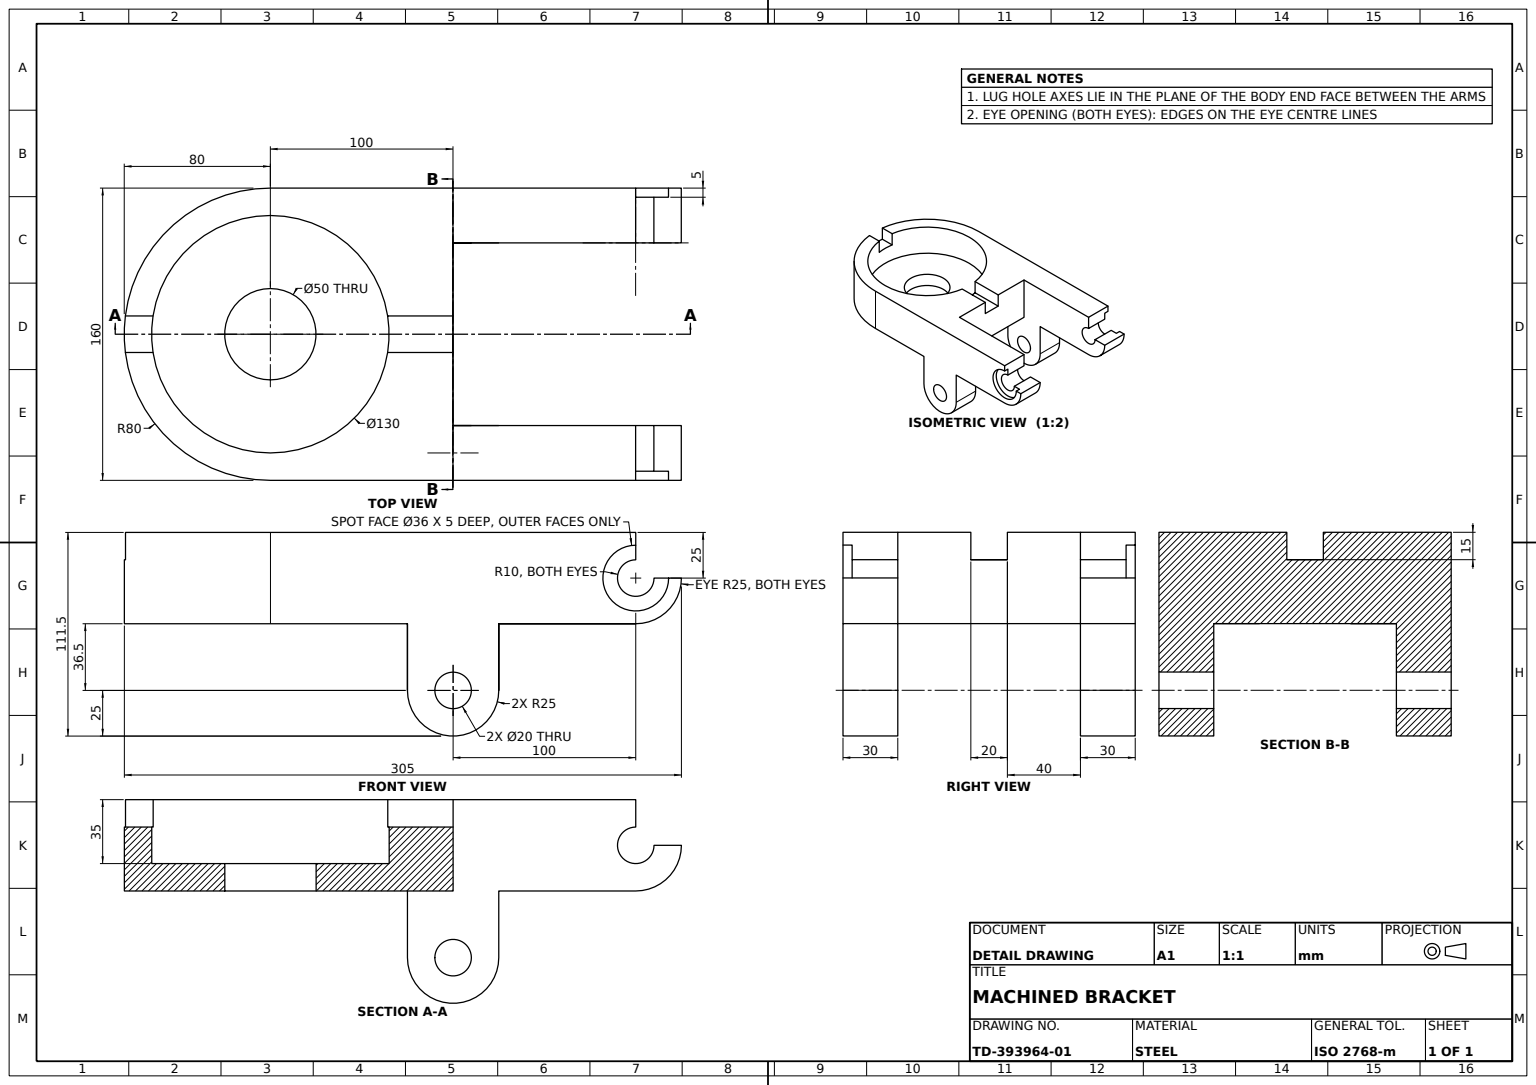
from build123d import *
from build123d.topology import SkipClean

# Parameters (mm, degrees)
BASE_PLATE_DEPTH                = 15
CIRCULAR_START                  = 35
CIRCULAR_HOUSING_DEPTH          = 35
HOUSING_EXTENSION_SKETCH_R      = 65
HOUSING_EXTENSION_SKETCH_R_2    = 25
HOUSING_EXTENSION_DEPTH         = 15
CLEVIS_LUG_BLOCK_SKETCH_R       = 25
CLEVIS_LUG_BLOCK_SKETCH_R_2     = 10
CLEVIS_LUG_BLOCK_DEPTH          = 30
CLEVIS_START                    = -30
CLEVIS_LUG_EXTENSION_SKETCH_R   = 25
CLEVIS_LUG_EXTENSION_SKETCH_R_2 = 10
CLEVIS_LUG_EXTENSION_DEPTH      = 30
PIVOT_LUG_SKETCH_R              = 25
PIVOT_LUGS_DEPTH                = 30
PIVOT_PIN_HOLE_SKETCH_R         = 10
PIVOT_PIN_HOLE_20_DEPTH         = 200
CLEVIS_SLOT_25_DEPTH            = 200
SPOT_FACE_A_SKETCH_R            = 18
SPOT_FACE_A_36X5_DEPTH          = 5
LUG_START                       = -30
LUG_FILL_BOSS_DEPTH             = 30
SPOT_START                      = -5
SPOT_FACE_B_SKETCH_R            = 18
SPOT_FACE_B_36X5_DEPTH          = 5


with BuildPart() as part:
    # Base Plate Sketch → Base Plate (new body)
    with BuildSketch(Plane(origin=(0, 0, 0), x_dir=(1, 0, 0), z_dir=(0, 1, 0))):
        with BuildLine():
            ThreePointArc((64.226162893, -10), (0, -65), (-64.226162893, -10))
            Line((-64.226162893, -10), (-79.372539332, -10))
            ThreePointArc((-79.372539332, -10), (-52.915026221, -60), (0, -80))
            ThreePointArc((0, -80), (52.915026221, -60), (79.372539332, -10))
            Line((79.372539332, -10), (64.226162893, -10))
        make_face()
        with BuildLine():
            ThreePointArc((0, 80), (-52.915026221, 60), (-79.372539332, 10))
            Line((-79.372539332, 10), (-64.226162893, 10))
            ThreePointArc((-64.226162893, 10), (0, 65), (64.226162893, 10))
            Line((64.226162893, 10), (79.372539332, 10))
            ThreePointArc((79.372539332, 10), (52.915026221, 60), (0, 80))
        make_face()
        with BuildLine():
            Line((200, 80), (0, 80))
            ThreePointArc((0, 80), (52.915026221, 60), (79.372539332, 10))
            Line((79.372539332, 10), (100, 10))
            Line((100, 10), (100, 50))
            Line((100, 50), (200, 50))
            Line((200, 50), (200, 80))
        make_face()
        with BuildLine():
            ThreePointArc((79.372539332, -10), (52.915026221, -60), (0, -80))
            Line((0, -80), (200, -80))
            Line((200, -80), (200, -50))
            Line((200, -50), (100, -50))
            Line((100, -50), (100, -10))
            Line((100, -10), (79.372539332, -10))
        make_face()
    extrude(amount=BASE_PLATE_DEPTH)

    # Circular Housing Sketch → Circular Housing (add)
    with BuildSketch(Plane.XZ.offset(CIRCULAR_START)):
        with BuildLine():
            ThreePointArc((79.372539332, 10), (52.915026221, 60), (0, 80))
            ThreePointArc((0, 80), (-52.915026221, 60), (-79.372539332, 10))
            Line((-79.372539332, 10), (-64.226162893, 10))
            ThreePointArc((-64.226162893, 10), (0, 65), (64.226162893, 10))
            Line((64.226162893, 10), (79.372539332, 10))
        make_face()
        with BuildLine():
            Line((-64.226162893, 10), (-79.372539332, 10))
            ThreePointArc((-79.372539332, 10), (-60, -52.915026221), (0, -80))
            ThreePointArc((0, -80), (56.568542495, -56.568542495), (80, 0))
            ThreePointArc((80, 0), (79.842980739, 5.009833003), (79.372539332, 10))
            Line((79.372539332, 10), (64.226162893, 10))
            ThreePointArc((64.226162893, 10), (64.806251967, 5.014948252), (65, 0))
            ThreePointArc((65, 0), (-5.014948252, -64.806251967), (-64.226162893, 10))
        make_face()
        with BuildLine():
            Line((200, 80), (0, 80))
            ThreePointArc((0, 80), (52.915026221, 60), (79.372539332, 10))
            Line((79.372539332, 10), (100, 10))
            Line((100, 10), (100, 50))
            Line((100, 50), (200, 50))
            Line((200, 50), (200, 80))
        make_face()
        with BuildLine():
            Line((100, 10), (79.372539332, 10))
            ThreePointArc((79.372539332, 10), (79.842980739, 5.009833003), (80, 0))
            ThreePointArc((80, 0), (56.568542495, -56.568542495), (0, -80))
            Line((0, -80), (200, -80))
            Line((200, -80), (200, -50))
            Line((200, -50), (100, -50))
            Line((100, -50), (100, 10))
        make_face()
    extrude(amount=-CIRCULAR_HOUSING_DEPTH)

    # Housing Extension Sketch → Housing Extension (add)
    with BuildSketch(Plane.XZ.offset(35)):
        with Locations(Location((0, 0, 0), (0, 0, 270))):
            Circle(HOUSING_EXTENSION_SKETCH_R)
        with Locations(Location((0, 0, 0), (0, 0, 270))):
            Circle(HOUSING_EXTENSION_SKETCH_R_2, mode=Mode.SUBTRACT)
    extrude(amount=-HOUSING_EXTENSION_DEPTH)

    # Clevis Lug Block Sketch → Clevis Lug Block (add)
    # profile 1 of 2: a face of its own
    with SkipClean():  # the faces are left unmerged after this step: merging them gives an invalid solid
        with BuildSketch(Plane.XY.offset(80)):
            with BuildLine():
                Line((75, -35), (75, -71.5))
                ThreePointArc((75, -71.5), (100, -46.5), (125, -71.5))
                Line((125, -71.5), (125, -35))
                Line((125, -35), (75, -35))
            make_face()
        # profile 2 of 2: a face of its own
        with BuildSketch(Plane.XY.offset(80)):
            with Locations((100, -71.5)):
                Circle(CLEVIS_LUG_BLOCK_SKETCH_R)
            with Locations((100, -71.5)):
                Circle(CLEVIS_LUG_BLOCK_SKETCH_R_2, mode=Mode.SUBTRACT)
        extrude(amount=-CLEVIS_LUG_BLOCK_DEPTH)

    # Clevis Lug Extension Sketch → Clevis Lug Extension (add)
    # profile 1 of 2: a face of its own
    with SkipClean():  # the faces are left unmerged after this step: merging them gives an invalid solid
        with BuildSketch(Plane(origin=(0, 0, -80), x_dir=(-1, 0, 0), z_dir=(0, 0, -1)).offset(CLEVIS_START)):
            with BuildLine():
                Line((-125, -35), (-125, -71.5))
                ThreePointArc((-125, -71.5), (-100, -46.5), (-75, -71.5))
                Line((-75, -71.5), (-75, -35))
                Line((-75, -35), (-125, -35))
            make_face()
        # profile 2 of 2: a face of its own
        with BuildSketch(Plane(origin=(0, 0, -80), x_dir=(-1, 0, 0), z_dir=(0, 0, -1)).offset(CLEVIS_START)):
            with Locations((-100, -71.5)):
                Circle(CLEVIS_LUG_EXTENSION_SKETCH_R)
            with Locations(Location((-100, -71.5, 0), (0, 0, 180))):
                Circle(CLEVIS_LUG_EXTENSION_SKETCH_R_2, mode=Mode.SUBTRACT)
        extrude(amount=CLEVIS_LUG_EXTENSION_DEPTH)

    # Pivot Lug Sketch → Pivot Lugs (add)
    with SkipClean():  # the faces are left unmerged after this step: merging them gives an invalid solid
        with BuildSketch(Plane.XY.offset(80)):
            with Locations((200, -10)):
                Circle(PIVOT_LUG_SKETCH_R)
        extrude(amount=-PIVOT_LUGS_DEPTH)

    # Pivot Pin Hole Sketch → Pivot Pin Hole Ø20 (cut)
    with SkipClean():  # the faces are left unmerged after this step: merging them gives an invalid solid
        with BuildSketch(Plane.XY.offset(80)):
            with Locations((200, -10)):
                Circle(PIVOT_PIN_HOLE_SKETCH_R)
        extrude(amount=-PIVOT_PIN_HOLE_20_DEPTH, mode=Mode.SUBTRACT)

    # Clevis Slot Sketch → Clevis Slot 25 (cut)
    with SkipClean():  # the faces are left unmerged after this step: merging them gives an invalid solid
        with BuildSketch(Plane.XY.offset(80)):
            with BuildLine():
                Line((200, 15), (200, -10))
                Line((200, -10), (225, -10))
                ThreePointArc((225, -10), (217.67766953, 7.67766953), (200, 15))
            make_face()
        extrude(amount=-CLEVIS_SLOT_25_DEPTH, mode=Mode.SUBTRACT)

    # Spot Face A Sketch → Spot Face A Ø36x5 (cut)
    with SkipClean():  # the faces are left unmerged after this step: merging them gives an invalid solid
        with BuildSketch(Plane.XY.offset(80)):
            with Locations((200, -10)):
                Circle(SPOT_FACE_A_SKETCH_R)
        extrude(amount=-SPOT_FACE_A_36X5_DEPTH, mode=Mode.SUBTRACT)

    # Lug Fill Sketch → Lug Fill Boss (add)
    with SkipClean():  # the faces are left unmerged after this step: merging them gives an invalid solid
        with BuildSketch(Plane(origin=(0, 0, -80), x_dir=(-1, 0, 0), z_dir=(0, 0, -1)).offset(LUG_START)):
            with BuildLine():
                Line((-210, -10), (-225, -10))
                ThreePointArc((-225, -10), (-217.67766953, -27.67766953), (-200, -35))
                Line((-200, -35), (-200, -20))
                ThreePointArc((-200, -20), (-207.071067812, -17.071067812), (-210, -10))
            make_face()
        extrude(amount=LUG_FILL_BOSS_DEPTH)

    # Spot Face B Sketch → Spot Face B Ø36x5 (cut)
    with SkipClean():  # the faces are left unmerged after this step: merging them gives an invalid solid
        with BuildSketch(Plane(origin=(0, 0, -80), x_dir=(-1, 0, 0), z_dir=(0, 0, -1)).offset(SPOT_START)):
            with Locations((-200, -10)):
                Circle(SPOT_FACE_B_SKETCH_R)
        extrude(amount=SPOT_FACE_B_36X5_DEPTH, mode=Mode.SUBTRACT)


solid = part.part
